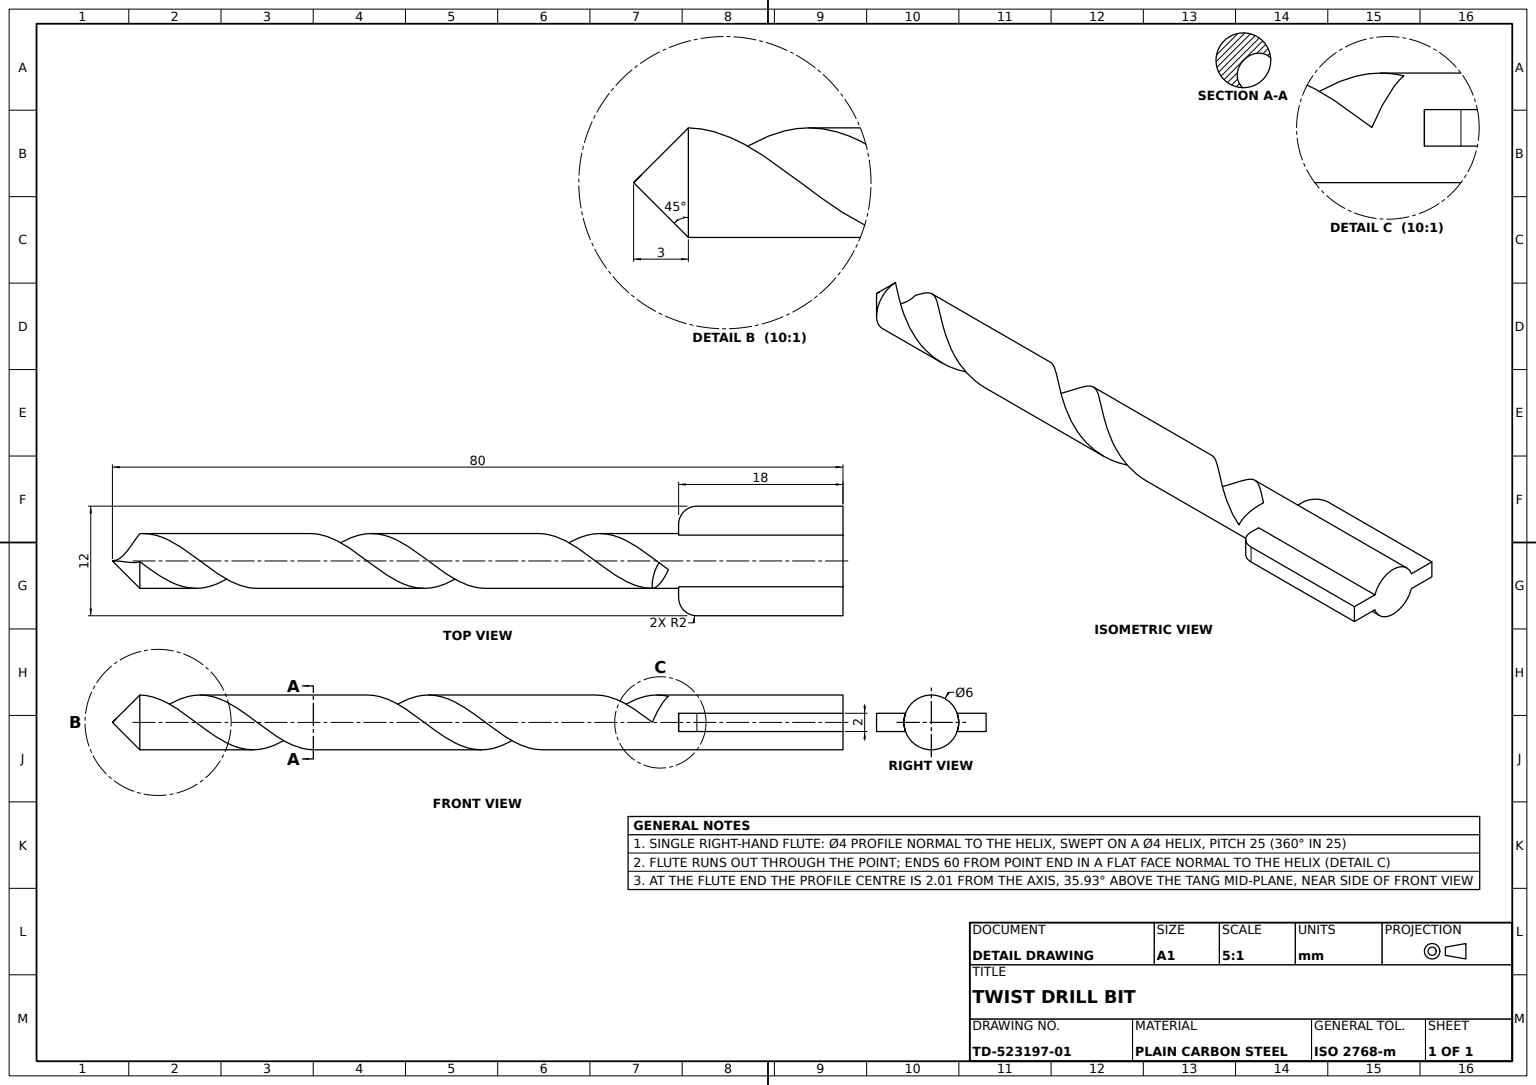
from build123d import *

# Parameters (mm, degrees)
BODY_PROFILE_6_R          = 3
DRILL_BODY_6_X_80_DEPTH   = 80
TIP_CHAMFER_3X45_SIZE     = 3
HELICAL_FLUTE_PITCH       = 25
HELICAL_FLUTE_HEIGHT      = 60
HELICAL_FLUTE_RADIUS      = 2
HELICAL_FLUTE_START_ANGLE = 180
FLUTE_PROFILE_4_R         = 2
TANG_PROFILE_12X18_W      = 12
TANG_PROFILE_12X18_H      = 18
DRIVE_TANG_2MM_DEPTH      = 1
TANG_FILLET_R2_A_R        = 2
TANG_FILLET_R2_B_R        = 2


with BuildPart() as part:
    # Body Profile Ø6 → Drill Body Ø6 x 80 (new body)
    with BuildSketch(Plane(origin=(0, 0, 0), x_dir=(1, 0, 0), z_dir=(0, 1, 0))):
        with Locations(Location((0, 0, 0), (0, 0, 270))):
            Circle(BODY_PROFILE_6_R)
    extrude(amount=DRILL_BODY_6_X_80_DEPTH)

    # Tip Chamfer 3x45°
    tip_chamfer_3x45_edges = [part.edges().sort_by_distance(p)[0] for p in [
        (0, 80, -3),
    ]]
    chamfer(tip_chamfer_3x45_edges, length=TIP_CHAMFER_3X45_SIZE)

    # Helical Flute: sweep along a helix
    with BuildLine() as helical_flute_path:
        add(Helix(HELICAL_FLUTE_PITCH, HELICAL_FLUTE_HEIGHT, HELICAL_FLUTE_RADIUS, center=(0, 80, 0), direction=(0, -1, 0), mode=Mode.PRIVATE).rotate(Axis((0, 80, 0), (0, -1, 0)), HELICAL_FLUTE_START_ANGLE))
    # Flute Profile Ø4 → Helical Flute (sweep, cut)
    with BuildSketch(Plane(origin=(0, 80, 2), x_dir=(-0.8934763687940476, 0.4491102074175148, -3.3349691128186272e-15), z_dir=(-0.44911020741751484, -0.8934763687940477, 6.634710242048462e-15))):
        with Locations((-0.000268006, -0.010109249)):
            Circle(FLUTE_PROFILE_4_R)
    sweep(path=helical_flute_path.line, is_frenet=True, mode=Mode.SUBTRACT)

    # Tang Profile 12x18 → Drive Tang 2mm (add, symmetric)
    with BuildSketch(Plane(origin=(0, 0, 0), x_dir=(0, 0, -1), z_dir=(1, 0, 0))):
        with Locations((0, 9)):
            Rectangle(TANG_PROFILE_12X18_W, TANG_PROFILE_12X18_H)
    extrude(amount=DRIVE_TANG_2MM_DEPTH, both=True)

    # Tang Fillet R2 A
    tang_fillet_r2_a_edges = [part.edges().sort_by_distance(p)[0] for p in [
        (0, 18, 6),
    ]]
    fillet(tang_fillet_r2_a_edges, radius=TANG_FILLET_R2_A_R)

    # Tang Fillet R2 B
    tang_fillet_r2_b_edges = [part.edges().sort_by_distance(p)[0] for p in [
        (0, 18, -6),
    ]]
    fillet(tang_fillet_r2_b_edges, radius=TANG_FILLET_R2_B_R)


solid = part.part
